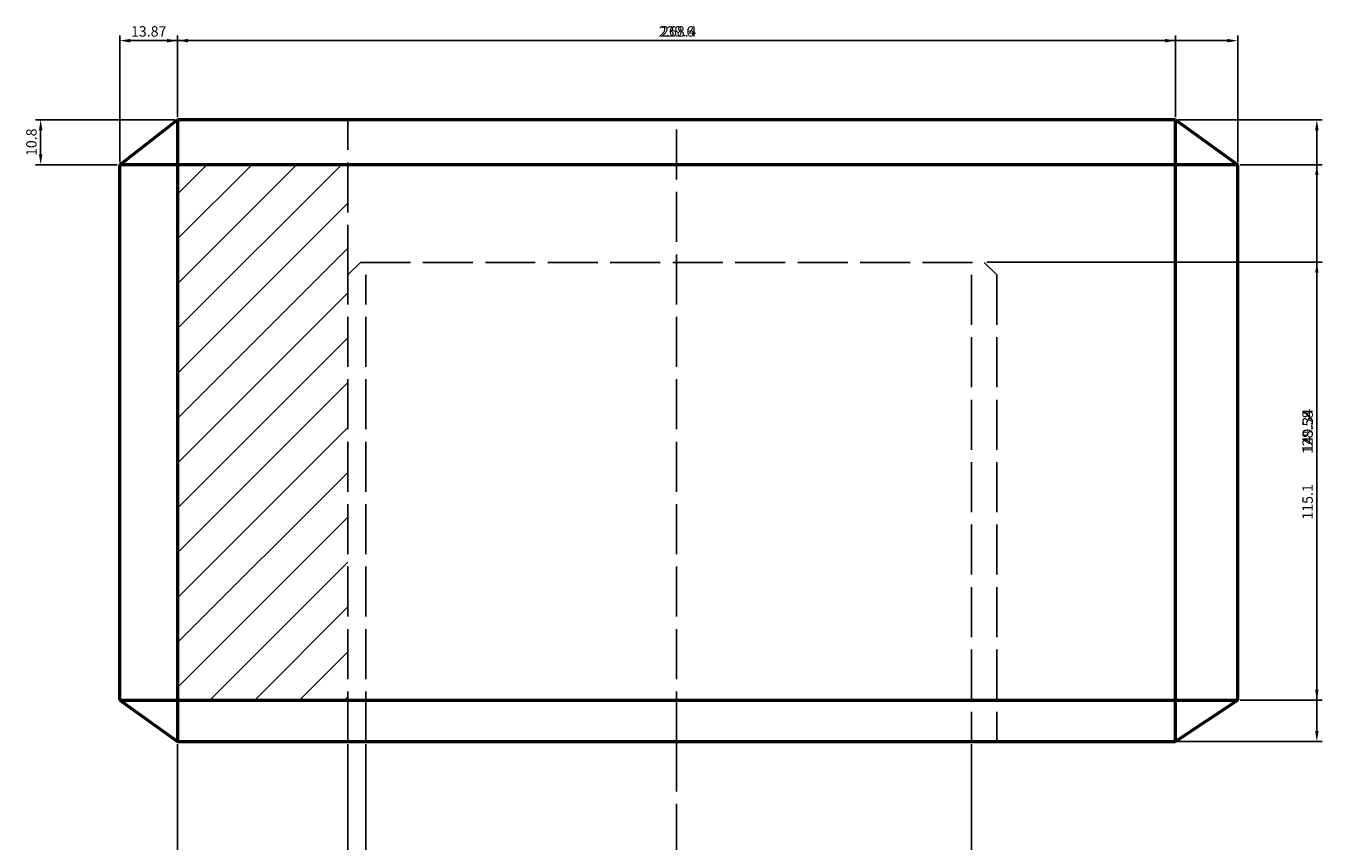
# Model space of a CAD drawing. Units: millimetres. Extents: x 921 to 2648, y 1390 to 2315.
# Tile 9 of 10: x 2291 to 2602, y 1719 to 1915. Entities that reach past the tile are written whole.
import ezdxf

# ---------------------------------------------------------------- set-up
doc = ezdxf.new("R2010")
doc.units = ezdxf.units.MM
doc.linetypes.add('ACAD_ISO02W100', pattern=[15, 12, -3])
for name, color, linetype, lineweight in [('M-DIMS', 2, 'Continuous', 25), ('M-HATC', 8, 'Continuous', 18), ('M-HIDN', 4, 'ACAD_ISO02W100', 25), ('M-OUTL', 7, 'Continuous', 50)]:
    doc.layers.add(name, color=color, linetype=linetype, lineweight=lineweight)
doc.styles.get("Standard").update_dxf_attribs({"font": 'arial.ttf'})
doc.dimstyles.new('ISO-25', dxfattribs={"dimtxt": 2.5, "dimasz": 2.5, "dimexe": 1.25, "dimexo": 0.625, "dimtad": 1, "dimtxsty": 'Standard', "dimcen": 2.5, "dimadec": 0, "dimazin": 0, "dimtfac": 1, "dimtmove": 0, "dimatfit": 3, "dimfxl": 1, "dimarcsym": 0})

# ---------------------------------------------------------------- blocks, each defined once
blk = doc.blocks.new('*D35')
at = {"layer": 'Defpoints', "color": 0, "transparency": 16777216}
for p in [(2582.04, 1881.91), (2582.04, 1753.32), (2601.04, 1753.32)]:
    blk.add_point(p, dxfattribs=at)
at = {"layer": 'M-DIMS', "color": 0, "lineweight": -2, "transparency": 16777216}
for p, q in [((2582.66, 1881.91), (2602.29, 1881.91)), ((2601.04, 1879.41), (2601.04, 1755.82)), ((2582.66, 1753.32), (2602.29, 1753.32))]:
    blk.add_line(p, q, dxfattribs=at)
at = {"layer": 'M-DIMS', "color": 0, "transparency": 16777216}
for points in [[(2600.62, 1879.41), (2601.45, 1879.41), (2601.04, 1881.91)], [(2600.62, 1755.82), (2601.45, 1755.82), (2601.04, 1753.32)]]:
    blk.add_solid(points, dxfattribs=at)
at = {"layer": 'M-DIMS', "color": 0, "transparency": 16777216, "insert": (2599.14, 1817.62), "char_height": 2.5, "attachment_point": 5, "rotation": 90}
blk.add_mtext('128.58', dxfattribs=at)
blk = doc.blocks.new('*D36')
at = {"layer": 'Defpoints', "color": 0, "transparency": 16777216}
for p in [(2567.1, 1911.71), (2327.48, 1892.71), (2567.1, 1892.71)]:
    blk.add_point(p, dxfattribs=at)
at = {"layer": 'M-DIMS', "color": 0, "lineweight": -2, "transparency": 16777216}
for p, q in [((2327.48, 1893.34), (2327.48, 1912.96)), ((2329.98, 1911.71), (2564.6, 1911.71)), ((2567.1, 1893.34), (2567.1, 1912.96))]:
    blk.add_line(p, q, dxfattribs=at)
at = {"layer": 'M-DIMS', "color": 0, "transparency": 16777216}
for points in [[(2329.98, 1912.13), (2329.98, 1911.29), (2327.48, 1911.71)], [(2564.6, 1912.13), (2564.6, 1911.29), (2567.1, 1911.71)]]:
    blk.add_solid(points, dxfattribs=at)
at = {"layer": 'M-DIMS', "color": 0, "transparency": 16777216, "insert": (2447.29, 1913.61), "char_height": 2.5, "attachment_point": 5}
blk.add_mtext('239.6', dxfattribs=at)
blk = doc.blocks.new('*D91')
at = {"layer": 'Defpoints', "color": 0, "transparency": 16777216}
for p in [(2327.48, 1911.71), (2327.48, 1892.71), (2313.61, 1881.91)]:
    blk.add_point(p, dxfattribs=at)
at = {"layer": 'M-DIMS', "color": 0, "lineweight": -2, "transparency": 16777216}
for p, q in [((2313.61, 1882.53), (2313.61, 1912.96)), ((2316.11, 1911.71), (2324.98, 1911.71)), ((2327.48, 1893.34), (2327.48, 1912.96))]:
    blk.add_line(p, q, dxfattribs=at)
at = {"layer": 'M-DIMS', "color": 0, "transparency": 16777216}
for points in [[(2316.11, 1912.13), (2316.11, 1911.29), (2313.61, 1911.71)], [(2324.98, 1912.13), (2324.98, 1911.29), (2327.48, 1911.71)]]:
    blk.add_solid(points, dxfattribs=at)
at = {"layer": 'M-DIMS', "color": 0, "transparency": 16777216, "insert": (2320.55, 1913.61), "char_height": 2.5, "attachment_point": 5}
blk.add_mtext('13.87', dxfattribs=at)
blk = doc.blocks.new('*D92')
at = {"layer": 'Defpoints', "color": 0, "transparency": 16777216}
for p in [(2294.61, 1892.71), (2327.48, 1892.71), (2313.61, 1881.91)]:
    blk.add_point(p, dxfattribs=at)
at = {"layer": 'M-DIMS', "color": 0, "lineweight": -2, "transparency": 16777216}
for p, q in [((2326.86, 1892.71), (2293.36, 1892.71)), ((2294.61, 1884.41), (2294.61, 1890.21)), ((2312.99, 1881.91), (2293.36, 1881.91))]:
    blk.add_line(p, q, dxfattribs=at)
at = {"layer": 'M-DIMS', "color": 0, "transparency": 16777216}
for points in [[(2294.2, 1890.21), (2295.03, 1890.21), (2294.61, 1892.71)], [(2294.2, 1884.41), (2295.03, 1884.41), (2294.61, 1881.91)]]:
    blk.add_solid(points, dxfattribs=at)
at = {"layer": 'M-DIMS', "color": 0, "transparency": 16777216, "insert": (2292.71, 1887.31), "char_height": 2.5, "attachment_point": 5, "rotation": 90}
blk.add_mtext('10.8', dxfattribs=at)
blk = doc.blocks.new('*D93')
at = {"layer": 'Defpoints', "color": 0, "transparency": 16777216}
for p in [(2582.04, 1911.71), (2313.61, 1881.91), (2582.04, 1881.91)]:
    blk.add_point(p, dxfattribs=at)
at = {"layer": 'M-DIMS', "color": 0, "lineweight": -2, "transparency": 16777216}
for p, q in [((2313.61, 1882.53), (2313.61, 1912.96)), ((2316.11, 1911.71), (2579.54, 1911.71)), ((2582.04, 1882.53), (2582.04, 1912.96))]:
    blk.add_line(p, q, dxfattribs=at)
at = {"layer": 'M-DIMS', "color": 0, "transparency": 16777216}
for points in [[(2316.11, 1912.13), (2316.11, 1911.29), (2313.61, 1911.71)], [(2579.54, 1912.13), (2579.54, 1911.29), (2582.04, 1911.71)]]:
    blk.add_solid(points, dxfattribs=at)
at = {"layer": 'M-DIMS', "color": 0, "transparency": 16777216, "insert": (2447.83, 1913.61), "char_height": 2.5, "attachment_point": 5}
blk.add_mtext('268.4', dxfattribs=at)
blk = doc.blocks.new('*D94')
at = {"layer": 'Defpoints', "color": 0, "transparency": 16777216}
for p in [(2567.1, 1892.71), (2567.1, 1743.37), (2601.04, 1743.37)]:
    blk.add_point(p, dxfattribs=at)
at = {"layer": 'M-DIMS', "color": 0, "lineweight": -2, "transparency": 16777216}
for p, q in [((2567.73, 1892.71), (2602.29, 1892.71)), ((2601.04, 1890.21), (2601.04, 1745.87)), ((2567.73, 1743.37), (2602.29, 1743.37))]:
    blk.add_line(p, q, dxfattribs=at)
at = {"layer": 'M-DIMS', "color": 0, "transparency": 16777216}
for points in [[(2600.62, 1890.21), (2601.45, 1890.21), (2601.04, 1892.71)], [(2600.62, 1745.87), (2601.45, 1745.87), (2601.04, 1743.37)]]:
    blk.add_solid(points, dxfattribs=at)
at = {"layer": 'M-DIMS', "color": 0, "transparency": 16777216, "insert": (2599.14, 1818.04), "char_height": 2.5, "attachment_point": 5, "rotation": 90}
blk.add_mtext('149.34', dxfattribs=at)
blk = doc.blocks.new('*D95')
at = {"layer": 'Defpoints', "color": 0, "transparency": 16777216}
for p in [(2327.48, 1743.37), (2368.38, 1743.37), (2368.38, 1518.64)]:
    blk.add_point(p, dxfattribs=at)
at = {"layer": 'M-DIMS', "color": 0, "lineweight": -2, "transparency": 16777216}
for p, q in [((2327.48, 1742.75), (2327.48, 1517.39)), ((2368.38, 1742.75), (2368.38, 1517.39)), ((2329.98, 1518.64), (2365.88, 1518.64))]:
    blk.add_line(p, q, dxfattribs=at)
at = {"layer": 'M-DIMS', "color": 0, "transparency": 16777216}
for points in [[(2329.98, 1519.05), (2329.98, 1518.22), (2327.48, 1518.64)], [(2365.88, 1519.05), (2365.88, 1518.22), (2368.38, 1518.64)]]:
    blk.add_solid(points, dxfattribs=at)
at = {"layer": 'M-DIMS', "color": 0, "transparency": 16777216, "insert": (2347.93, 1520.54), "char_height": 2.5, "attachment_point": 5}
blk.add_mtext('40.9', dxfattribs=at)
blk = doc.blocks.new('*D96')
at = {"layer": 'Defpoints', "color": 0, "transparency": 16777216}
for p in [(2372.67, 1743.37), (2518.1, 1743.37), (2518.1, 1518.64)]:
    blk.add_point(p, dxfattribs=at)
at = {"layer": 'M-DIMS', "color": 0, "lineweight": -2, "transparency": 16777216}
for p, q in [((2372.67, 1742.75), (2372.67, 1517.39)), ((2518.1, 1742.75), (2518.1, 1517.39)), ((2375.17, 1518.64), (2515.6, 1518.64))]:
    blk.add_line(p, q, dxfattribs=at)
at = {"layer": 'M-DIMS', "color": 0, "transparency": 16777216}
for points in [[(2375.17, 1519.05), (2375.17, 1518.22), (2372.67, 1518.64)], [(2515.6, 1519.05), (2515.6, 1518.22), (2518.1, 1518.64)]]:
    blk.add_solid(points, dxfattribs=at)
at = {"layer": 'M-DIMS', "color": 0, "transparency": 16777216, "insert": (2445.38, 1520.54), "char_height": 2.5, "attachment_point": 5}
blk.add_mtext('145.43', dxfattribs=at)
blk = doc.blocks.new('*D97')
at = {"layer": 'Defpoints', "color": 0, "transparency": 16777216}
for p in [(2521.18, 1858.47), (2524.18, 1743.37), (2601.04, 1743.37)]:
    blk.add_point(p, dxfattribs=at)
at = {"layer": 'M-DIMS', "color": 0, "lineweight": -2, "transparency": 16777216}
for p, q in [((2521.81, 1858.47), (2602.29, 1858.47)), ((2601.04, 1855.97), (2601.04, 1745.87)), ((2524.81, 1743.37), (2602.29, 1743.37))]:
    blk.add_line(p, q, dxfattribs=at)
at = {"layer": 'M-DIMS', "color": 0, "transparency": 16777216}
for points in [[(2600.62, 1855.97), (2601.45, 1855.97), (2601.04, 1858.47)], [(2600.62, 1745.87), (2601.45, 1745.87), (2601.04, 1743.37)]]:
    blk.add_solid(points, dxfattribs=at)
at = {"layer": 'M-DIMS', "color": 0, "transparency": 16777216, "insert": (2599.14, 1800.92), "char_height": 2.5, "attachment_point": 5, "rotation": 90}
blk.add_mtext('115.1', dxfattribs=at)

msp = doc.modelspace()

# ---------------------------------------------------------------- hatches: boundary and pattern name
at = {"layer": 'M-HATC'}
h = msp.add_hatch(dxfattribs=at)
h.set_pattern_fill('ANSI31', color=256, scale=2.4)
h.paths.add_polyline_path([(2368.3795, 1855.4653), (2368.3795, 1881.9094), (2327.4822, 1881.9094), (2327.4822, 1753.3247), (2368.3795, 1753.3247)])

# ---------------------------------------------------------------- linework, layer by layer
at = {"layer": 'M-HIDN'}
for p, q in [((2368.3795, 1855.4653), (2368.3795, 1892.71)), ((2447.2926, 1743.373), (2447.2926, 1892.71)), ((2368.3795, 1855.4653), (2371.3795, 1858.4653)), ((2371.3795, 1858.4653), (2521.1836, 1858.4653)), ((2524.1836, 1855.4653), (2521.1836, 1858.4653)), ((2368.3795, 1743.373), (2368.3795, 1855.4653)), ((2372.6661, 1743.373), (2372.6661, 1855.4653)), ((2518.0959, 1855.4653), (2518.0959, 1743.373)), ((2524.1836, 1855.4653), (2524.1836, 1743.373)), ((2447.2926, 1743.373), (2447.2926, 1626.0228))]:
    msp.add_line(p, q, dxfattribs=at)
at = {"layer": 'M-OUTL'}
for p, q in [((2313.6123, 1881.9094), (2327.4822, 1892.71)), ((2567.1029, 1892.71), (2327.4822, 1892.71)), ((2327.4822, 1892.71), (2327.4822, 1743.373)), ((2567.1029, 1743.373), (2567.1029, 1892.71)), ((2567.1029, 1892.71), (2582.038, 1881.9094)), ((2582.038, 1881.9094), (2313.6123, 1881.9094)), ((2313.6123, 1753.3247), (2313.6123, 1881.9094)), ((2582.038, 1753.3247), (2582.038, 1881.9094)), ((2313.6123, 1753.3247), (2582.038, 1753.3247)), ((2313.6123, 1753.3247), (2327.4822, 1743.373)), ((2582.038, 1753.3247), (2567.1029, 1743.373)), ((2327.4822, 1743.373), (2567.1029, 1743.373)), ((2327.4822, 1743.373), (2327.4822, 1743.373))]:
    msp.add_line(p, q, dxfattribs=at)

# ---------------------------------------------------------------- dimensions: what is measured, and where the dimension line sits
at = {"layer": 'M-DIMS'}
for base, p1, p2, override, picture, middle in [((2327.4822, 1911.71), (2313.6123, 1881.9094), (2327.4822, 1892.71), {"dimdec": 2, "dimlfac": 1, "dimrnd": 0, "dimzin": 0, "dimdsep": 46, "dimlunit": 2}, '*D91', (2320.5473, 1913.6123)), ((2582.038, 1911.71), (2313.6123, 1881.9094), (2582.038, 1881.9094), {"dimdec": 1, "dimlfac": 1, "dimrnd": 0, "dimzin": 0, "dimdsep": 46, "dimlunit": 2}, '*D93', (2447.8252, 1913.6114)), ((2567.1029, 1911.71), (2327.4822, 1892.71), (2567.1029, 1892.71), {"dimdec": 1, "dimlfac": 1, "dimrnd": 0, "dimzin": 0, "dimdsep": 46, "dimlunit": 2}, '*D36', (2447.2926, 1913.6123)), ((2368.3795, 1518.6366), (2327.4822, 1743.373), (2368.3795, 1743.373), {"dimdec": 1, "dimlfac": 1, "dimrnd": 0, "dimzin": 0, "dimdsep": 46, "dimlunit": 2}, '*D95', (2347.9309, 1520.538)), ((2518.0959, 1518.6366), (2372.6661, 1743.373), (2518.0959, 1743.373), {"dimdec": 2, "dimlfac": 1, "dimrnd": 0, "dimzin": 0, "dimdsep": 46, "dimlunit": 2}, '*D96', (2445.381, 1520.5389))]:
    dim = msp.add_linear_dim(base=base, p1=p1, p2=p2, dimstyle='ISO-25', override=override, dxfattribs=at)
    dim.commit()
    dim.dimension.update_dxf_attribs({"geometry": picture, "text_midpoint": middle})
for base, p1, p2, override, picture, middle in [((2294.6123, 1892.71), (2313.6123, 1881.9094), (2327.4822, 1892.71), {"dimdec": 1, "dimlfac": 1, "dimrnd": 0, "dimzin": 0, "dimdsep": 46, "dimlunit": 2}, '*D92', (2292.7109, 1887.3097)), ((2601.038, 1743.373), (2567.1029, 1892.71), (2567.1029, 1743.373), {"dimdec": 2, "dimlfac": 1, "dimrnd": 0, "dimzin": 0, "dimdsep": 46, "dimlunit": 2}, '*D94', (2599.1357, 1818.0415)), ((2601.038, 1753.3247), (2582.038, 1881.9094), (2582.038, 1753.3247), {"dimdec": 2, "dimlfac": 1, "dimrnd": 0, "dimzin": 0, "dimdsep": 46, "dimlunit": 2}, '*D35', (2599.1366, 1817.6171)), ((2601.038, 1743.373), (2521.1836, 1858.4653), (2524.1836, 1743.373), {"dimdec": 1, "dimlfac": 1, "dimrnd": 0, "dimzin": 0, "dimdsep": 46, "dimlunit": 2}, '*D97', (2599.1366, 1800.9191))]:
    dim = msp.add_linear_dim(base=base, p1=p1, p2=p2, angle=90, dimstyle='ISO-25', override=override, dxfattribs=at)
    dim.commit()
    dim.dimension.update_dxf_attribs({"geometry": picture, "text_midpoint": middle})

doc.saveas('drawing.dxf')
